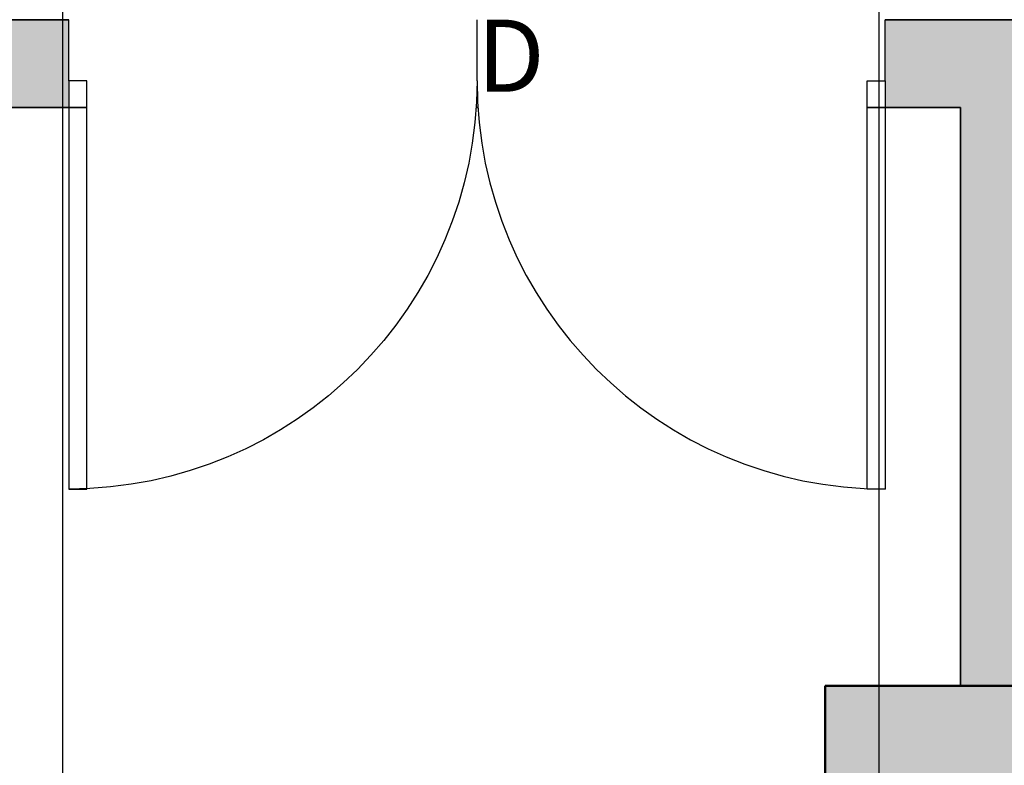
# Model space of a CAD drawing. Units: inches. Extents: x 1998 to 2588, y 1139 to 1977.
# Tile 39 of 134: x 2293 to 2344, y 1484 to 1523. Entities that reach past the tile are written whole.
import ezdxf

# ---------------------------------------------------------------- set-up
doc = ezdxf.new("R2010")
doc.units = ezdxf.units.IN
for name, color, linetype, lineweight in [('A-ANNO-DIMS', 2, 'Continuous', 18), ('A-COLS-PATT', 250, 'Continuous', 13), ('A-DOOR-IDEN', 7, 'Continuous', 18), ('A-WALL-PATT', 252, 'Continuous', 13), ('COLUMN', 10, 'Continuous', 50), ('DOOR', 52, 'Continuous', 25), ('WALL', 200, 'Continuous', 35)]:
    doc.layers.add(name, color=color, linetype=linetype, lineweight=lineweight)
doc.styles.get("Standard").update_dxf_attribs({"font": 'arial.ttf'})
doc.dimstyles.get("Standard").update_dxf_attribs({"dimtxt": 0.18, "dimasz": 0.18, "dimexe": 0.18, "dimexo": 0.0625, "dimgap": 0.09, "dimtad": 0, "dimtih": 1, "dimtoh": 1, "dimdec": 4, "dimzin": 0, "dimdsep": 46, "dimtxsty": 'Standard', "dimcen": 0.09, "dimadec": 0, "dimazin": 0, "dimtfac": 1, "dimtdec": 4, "dimtofl": 0, "dimtmove": 0, "dimatfit": 3, "dimfxl": 1, "dimtolj": 1, "dimtzin": 0, "dimarcsym": 0})

# ---------------------------------------------------------------- blocks, each defined once
blk = doc.blocks.new('*U2')
for p, q in [((0, 0), (0, -6)), ((40, 0), (40, -6))]:
    blk.add_line(p, q)
blk.add_lwpolyline([(0, 0), (0, 40), (1.75, 40), (1.75, 0)], close=True)
blk.add_arc((0, 0), 40, 0, 90)
blk = doc.blocks.new('*D44')
at = {"layer": 'A-ANNO-DIMS', "color": 0, "lineweight": -2, "transparency": 16777216}
for p, q in [((2295.414, 1588.67), (2295.414, 1138.602)), ((2337.287, 1588.67), (2337.287, 1138.602)), ((2295.594, 1138.782), (2315.953, 1138.782)), ((2337.107, 1138.782), (2316.748, 1138.782))]:
    blk.add_line(p, q, dxfattribs=at)
at = {"layer": 'A-ANNO-DIMS', "color": 0, "transparency": 16777216}
for points in [[(2295.594, 1138.812), (2295.594, 1138.752), (2295.414, 1138.782)], [(2337.107, 1138.812), (2337.107, 1138.752), (2337.287, 1138.782)]]:
    blk.add_solid(points, dxfattribs=at)
at = {"layer": 'Defpoints', "color": 0, "transparency": 16777216}
for p in [(2295.414, 1588.732), (2337.287, 1588.732), (2337.287, 1138.782)]:
    blk.add_point(p, dxfattribs=at)
at = {"layer": 'A-ANNO-DIMS', "color": 0, "transparency": 16777216, "insert": (2316.35, 1138.782), "char_height": 0.18, "attachment_point": 5}
blk.add_mtext('\\A1;41.87', dxfattribs=at)

msp = doc.modelspace()

# ---------------------------------------------------------------- hatches: boundary and pattern name
at = {"layer": 'A-COLS-PATT'}
h = msp.add_hatch(color=256, dxfattribs=at)
h.dxf.hatch_style = 1
h.paths.add_polyline_path([(2099.4125, 1888.7324), (2087.9729, 1888.7324), (2087.9729, 1868.3278), (2099.4125, 1868.3278)])
h.paths.add_polyline_path([(2234.4125, 1888.7324), (2222.9729, 1888.7324), (2222.9729, 1868.3278), (2234.4125, 1868.3278)])
h.paths.add_polyline_path([(2341.4729, 1886.637), (2330.0332, 1886.637), (2330.0332, 1866.2324), (2341.4729, 1866.2324)])
h.paths.add_polyline_path([(2507.8006, 1882.7324), (2487.396, 1882.7324), (2487.396, 1871.2927), (2507.8006, 1871.2927)])
h.paths.add_polyline_path([(2510.9729, 1766.672), (2490.5682, 1766.672), (2490.5682, 1755.2324), (2510.9729, 1755.2324)])
h.paths.add_polyline_path([(2345.9729, 1759.7324), (2334.5332, 1759.7324), (2334.5332, 1739.3278), (2345.9729, 1739.3278)])
h.paths.add_polyline_path([(2234.4125, 1774.3318), (2222.9729, 1774.3318), (2222.9729, 1753.9272), (2234.4125, 1753.9272)])
h.paths.add_polyline_path([(2099.4125, 1775.637), (2087.9729, 1775.637), (2087.9729, 1755.2324), (2099.4125, 1755.2324)])
h.paths.add_polyline_path([(2098.0956, 1593.7241), (2077.691, 1593.7241), (2077.691, 1582.2845), (2098.0956, 1582.2845)])
h.paths.add_polyline_path([(2227.4729, 1604.637), (2216.0332, 1604.637), (2216.0332, 1584.2324), (2227.4729, 1584.2324)])
h.paths.add_polyline_path([(2345.9729, 1647.5211), (2334.5332, 1647.5211), (2334.5332, 1627.1165), (2345.9729, 1627.1165)])
h.paths.add_polyline_path([(2522.3775, 1641.2324), (2501.9729, 1641.2324), (2501.9729, 1629.7927), (2522.3775, 1629.7927)])
h.paths.add_polyline_path([(2522.3775, 1480.7324), (2501.9729, 1480.7324), (2501.9729, 1469.2927), (2522.3775, 1469.2927)])
h.paths.add_polyline_path([(2345.9729, 1488.5616), (2334.5332, 1488.5616), (2334.5332, 1468.1569), (2345.9729, 1468.1569)])
h.paths.add_polyline_path([(2234.4125, 1486.137), (2227.4729, 1486.137), (2227.4729, 1465.7324), (2234.4125, 1465.7324)])
h.paths.add_polyline_path([(2227.4729, 1486.137), (2222.9729, 1486.137), (2222.9729, 1465.7324), (2227.4729, 1465.7324)])
h.paths.add_polyline_path([(2108.3775, 1470.2324), (2087.9729, 1470.2324), (2087.9729, 1458.7927), (2108.3775, 1458.7927)])
h.paths.add_polyline_path([(2096.9729, 1365.5012), (2087.9729, 1365.5012), (2087.9729, 1345.0966), (2096.9729, 1345.0966)])
h.paths.add_polyline_path([(2087.9729, 1365.5012), (2085.5332, 1365.5012), (2085.5332, 1345.0966), (2087.9729, 1345.0966)])
h.paths.add_polyline_path([(2234.4125, 1285.137), (2222.9729, 1285.137), (2222.9729, 1264.7324), (2234.4125, 1264.7324)])
h.paths.add_polyline_path([(2345.9729, 1285.137), (2334.5332, 1285.137), (2334.5332, 1264.7324), (2345.9729, 1264.7324)])
h.paths.add_polyline_path([(2503.1458, 1240.172), (2482.7412, 1240.172), (2482.7412, 1228.7324), (2503.1458, 1228.7324)])
h.paths.add_polyline_path([(2510.9729, 1369.172), (2490.5682, 1369.172), (2490.5682, 1357.7324), (2510.9729, 1357.7324)])
at = {"layer": 'A-WALL-PATT'}
h = msp.add_hatch(color=256, dxfattribs=at)
h.dxf.hatch_style = 1
h.paths.add_polyline_path([(2222.9729, 1888.7324), (2099.4125, 1888.7324), (2099.4125, 1879.7324), (2222.9729, 1879.7324)])
h.paths.add_polyline_path([(2096.9729, 1868.3278), (2087.9729, 1868.3278), (2087.9729, 1775.637), (2096.9729, 1775.637)])
h.paths.add_polyline_path([(2227.4729, 1868.3278), (2222.9729, 1868.3278), (2222.9729, 1774.3318), (2227.4729, 1774.3318)])
h.paths.add_polyline_path([(2188.3019, 1759.7324), (2138.6074, 1759.7324), (2099.4125, 1759.7324), (2099.4125, 1755.2324), (2176.9729, 1755.2324), (2188.3019, 1755.2324)])
h.paths.add_polyline_path([(2087.9729, 1759.7324), (2059.4729, 1759.7324), (2059.4729, 1702.7324), (2087.9729, 1702.7324), (2087.9729, 1707.2324), (2063.9729, 1707.2324), (2063.9729, 1755.2324), (2087.9729, 1755.2324)])
h.paths.add_polyline_path([(2096.9729, 1755.2324), (2087.9729, 1755.2324), (2087.9729, 1707.2324), (2096.9729, 1707.2324)])
h.paths.add_polyline_path([(2187.0461, 1707.2324), (2105.9729, 1707.2324), (2096.9729, 1707.2324), (2087.9729, 1707.2324), (2087.9729, 1702.7324), (2105.9729, 1702.7324), (2114.9729, 1702.7324), (2187.0461, 1702.7324)])
h.paths.add_polyline_path([(2181.4729, 1719.2028), (2176.9729, 1719.2028), (2176.9729, 1707.2324), (2181.4729, 1707.2324)])
h.paths.add_polyline_path([(2216.0332, 1588.7324), (2114.9729, 1588.7324), (2105.9729, 1588.7324), (2105.9729, 1584.2324), (2216.0332, 1584.2324)])
h.paths.add_polyline_path([(2077.691, 1588.7324), (2061.4729, 1588.7324), (2061.4729, 1584.2324), (2077.691, 1584.2324)])
h.paths.add_polyline_path([(2105.9729, 1588.7324), (2098.0956, 1588.7324), (2098.0956, 1584.2324), (2105.9729, 1584.2324)])
h.paths.add_polyline_path([(2114.9729, 1596.2642), (2110.1012, 1596.2642), (2105.9729, 1596.2642), (2105.9729, 1588.7324), (2114.9729, 1588.7324)])
h.paths.add_polyline_path([(2114.9729, 1584.2324), (2105.9729, 1584.2324), (2105.9729, 1580.249), (2110.1012, 1580.249), (2114.9729, 1580.249)])
h.paths.add_polyline_path([(2114.9729, 1547.7716), (2110.1012, 1547.7716, -0.0318759), (2105.9729, 1548.035), (2105.9729, 1470.2324), (2108.3775, 1470.2324), (2108.3775, 1465.7324), (2186.2943, 1465.7324), (2186.2943, 1470.2324), (2114.9729, 1470.2324)])
h.paths.add_polyline_path([(2227.4729, 1584.2324), (2222.9729, 1584.2324), (2222.9729, 1486.137), (2227.4729, 1486.137)])
h.paths.add_polyline_path([(2295.4138, 1593.2324), (2227.4729, 1593.2324), (2227.4729, 1588.7324), (2295.4138, 1588.7324), (2295.4138, 1591.8729)])
h.paths.add_polyline_path([(2345.9729, 1627.1165), (2341.4729, 1627.1165), (2341.4729, 1593.2324), (2337.2869, 1593.2324), (2337.2869, 1591.8729), (2337.2869, 1588.7324), (2345.9729, 1588.7324)])
h.paths.add_polyline_path([(2291.9729, 1588.7324), (2287.4729, 1588.7324), (2287.4729, 1522.7324), (2291.9729, 1522.7324)])
h.paths.add_polyline_path([(2291.9729, 1522.7324), (2287.4729, 1522.7324), (2227.4729, 1522.7324), (2227.4729, 1518.2324), (2291.9729, 1518.2324)])
h.paths.add_polyline_path([(2295.7347, 1519.5919), (2295.7347, 1522.7324), (2291.9729, 1522.7324), (2291.9729, 1518.2324), (2295.7347, 1518.2324)])
h.paths.add_polyline_path([(2345.9729, 1522.7324), (2337.6078, 1522.7324), (2337.6078, 1519.5919), (2337.6078, 1518.2324), (2341.4729, 1518.2324), (2341.4729, 1488.5616), (2345.9729, 1488.5616)])
h.paths.add_polyline_path([(2345.9729, 1468.1569), (2341.4729, 1468.1569), (2341.4729, 1374.2324), (2227.4729, 1374.2324), (2227.4729, 1369.7324), (2345.9729, 1369.7324)])
h.paths.add_polyline_path([(2345.9729, 1369.7324), (2341.4729, 1369.7324), (2341.4729, 1362.2324), (2345.9729, 1362.2324)])
h.paths.add_polyline_path([(2345.9729, 1317.7324), (2345.9729, 1322.2324), (2341.4729, 1322.2324), (2341.4729, 1285.137), (2345.9729, 1285.137)], flags=17)
h.paths.add_polyline_path([(2356.2096, 1322.2324), (2345.9729, 1322.2324), (2345.9729, 1317.7324), (2356.2096, 1317.7324), (2356.2096, 1319.3088)], flags=17)
h.paths.add_polyline_path([(2393.9729, 1322.2324), (2375.6999, 1322.2324), (2375.6999, 1319.3088, -0.0202458), (2375.636, 1317.7324), (2393.9729, 1317.7324)], flags=17)
h.paths.add_polyline_path([(2398.4729, 1322.2324), (2393.9729, 1322.2324), (2393.9729, 1317.7324), (2393.9729, 1237.7324), (2345.9729, 1237.7324), (2345.9729, 1264.7324), (2341.4729, 1264.7324), (2341.4729, 1228.7324), (2393.9729, 1228.7324), (2482.7412, 1228.7324), (2482.7412, 1237.7324), (2398.4729, 1237.7324), (2398.4729, 1297.1029)])
h.paths.add_polyline_path([(2398.4729, 1362.2324), (2393.9729, 1362.2324), (2393.9729, 1357.7324), (2398.4729, 1357.7324)])
h.paths.add_polyline_path([(2345.9729, 1329.7549), (2341.4729, 1329.7549), (2341.4729, 1322.2324), (2345.9729, 1322.2324)])

# ---------------------------------------------------------------- linework, layer by layer
at = {"layer": 'COLUMN'}
msp.add_lwpolyline([(2334.5332, 1488.5616), (2345.9729, 1488.5616), (2345.9729, 1468.1569), (2334.5332, 1468.1569)], close=True, dxfattribs=at)
at = {"layer": 'WALL'}
for p, q in [((2227.4729, 1522.7324), (2295.7347, 1522.7324)), ((2337.6078, 1522.7324), (2345.9729, 1522.7324)), ((2227.4729, 1518.2324), (2296.6507, 1518.2324)), ((2316.6271, 1518.2324), (2316.7155, 1518.2324)), ((2336.6919, 1518.2324), (2341.4729, 1518.2324)), ((2341.4729, 1518.2324), (2341.4729, 1488.5616))]:
    msp.add_line(p, q, dxfattribs=at)

# ---------------------------------------------------------------- block references
at = {"layer": 'DOOR', "yscale": 0.5234138920659225, "zscale": 0.5234138920659225, "rotation": 180}
for p, xscale in [((2295.7347, 1519.5919), -0.5234138920659225), ((2337.6078, 1519.5919), 0.5234138920659225)]:
    msp.add_blockref('*U2', p, dxfattribs=dict(at, xscale=xscale))

# ---------------------------------------------------------------- texts
at = {"layer": 'A-DOOR-IDEN', "insert": (2316.6713, 1522.7324), "char_height": 3.6988, "attachment_point": 1}
msp.add_mtext_dynamic_manual_height_columns('D', width=110.572713, gutter_width=18.4938, heights=[0], dxfattribs=at)

# ---------------------------------------------------------------- dimensions: what is measured, and where the dimension line sits
at = {"layer": 'A-ANNO-DIMS'}
dim = msp.add_linear_dim(base=(2337.2869, 1138.7824), p1=(2295.4138, 1588.7324), p2=(2337.2869, 1588.7324), dimstyle='Standard', override={"dimdec": 2, "dimlfac": 1, "dimrnd": 0, "dimzin": 0, "dimdsep": 46, "dimlunit": 2}, dxfattribs=at)
dim.commit()
dim.dimension.update_dxf_attribs({"geometry": '*D44', "text_midpoint": (2316.3503, 1138.7824)})

doc.saveas('drawing.dxf')
